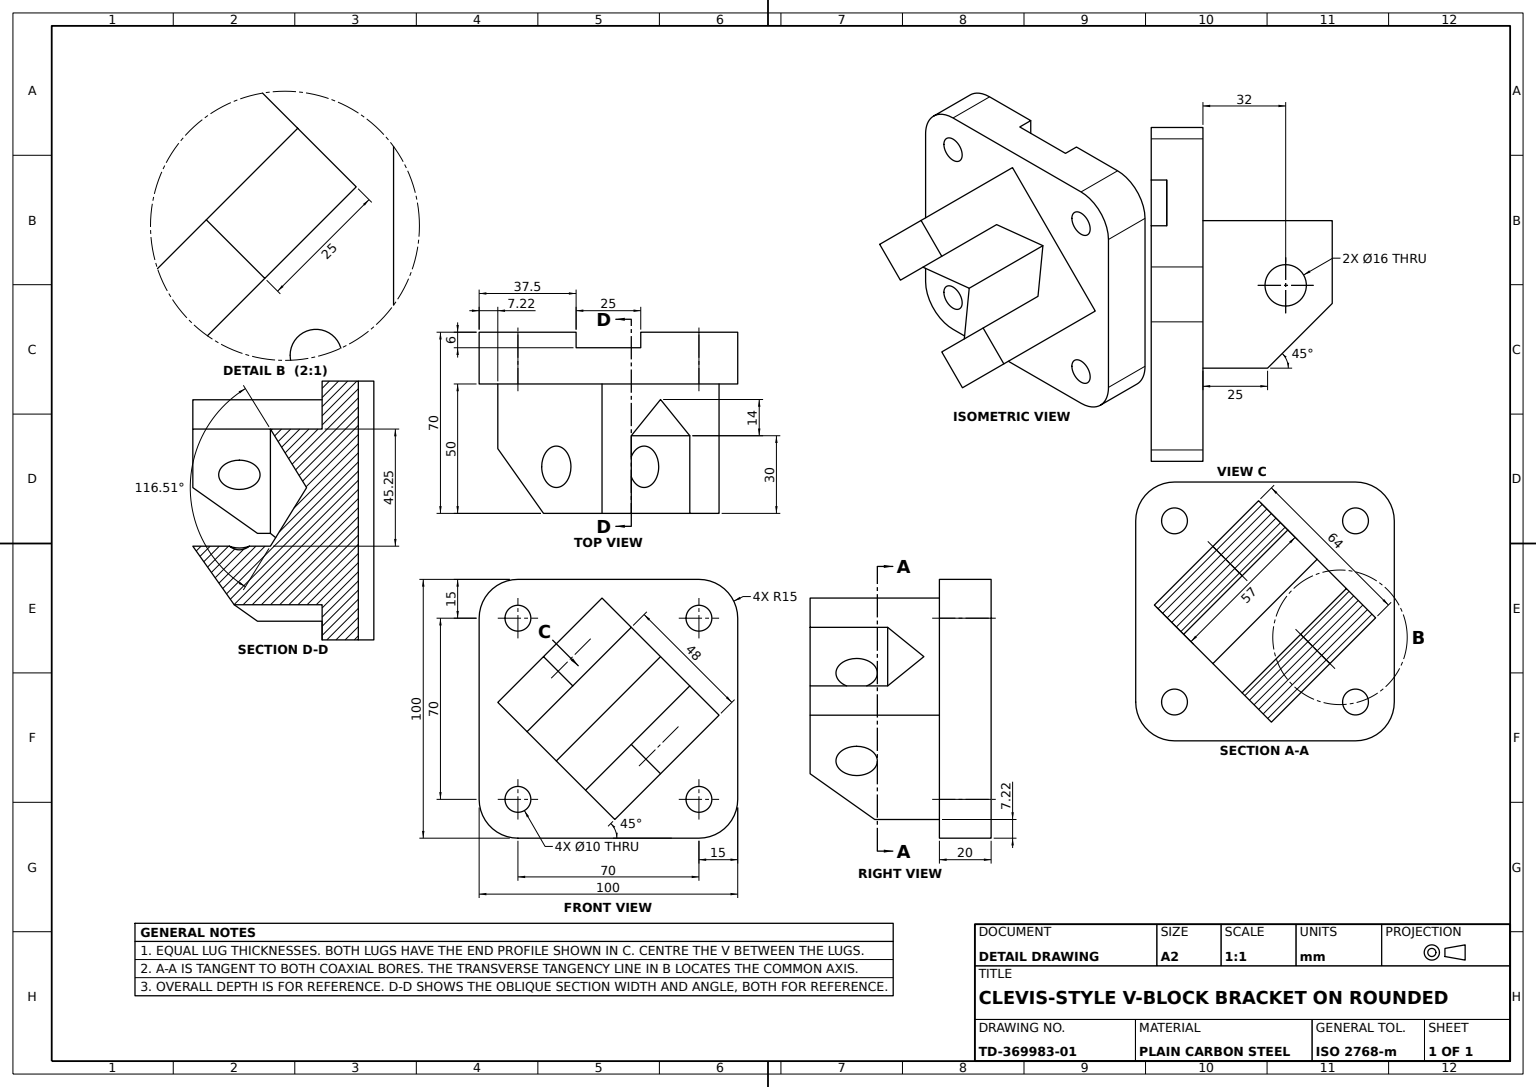
from build123d import *

# Parameters (mm, degrees)
BASE_PLATE_SKETCH_R       = 5
BASE_PLATE_DEPTH          = 20
PLATE_HOLES_12_DEPTH      = 114.578166916
PLATE_HOLES_12_DEPTH_BACK = 114.578166916
PLATE_HOLES_SKETCH_W      = 25
PLATE_HOLES_SKETCH_H      = 12
SQUARE_BOSS_DEPTH         = 50
BOSS_HOLE_16_DEPTH        = 125.295950858
BOSS_HOLE_16_DEPTH_BACK   = 125.295950858
BOSS_HOLE_SKETCH_R        = 8
BOSS_CHAMFER_25X45_SIZE   = 25
SLOT_CUT_DEPTH            = 122.4197622
SLOT_CUT_DEPTH_BACK       = 122.4197622


with BuildPart() as part:
    # Base Plate Sketch → Base Plate (new body)
    with BuildSketch(Plane.XY):
        with BuildLine():
            Line((-35, 50), (35, 50))
            ThreePointArc((35, 50), (45.606601718, 45.606601718), (50, 35))
            Line((50, 35), (50, -35))
            ThreePointArc((50, -35), (45.606601718, -45.606601718), (35, -50))
            Line((35, -50), (-35, -50))
            ThreePointArc((-35, -50), (-45.606601718, -45.606601718), (-50, -35))
            Line((-50, -35), (-50, 35))
            ThreePointArc((-50, 35), (-45.606601718, 45.606601718), (-35, 50))
        make_face()
        with Locations((-35, 35)):
            Circle(BASE_PLATE_SKETCH_R, mode=Mode.SUBTRACT)
        with Locations((35, 35)):
            Circle(BASE_PLATE_SKETCH_R, mode=Mode.SUBTRACT)
        with Locations((35, -35)):
            Circle(BASE_PLATE_SKETCH_R, mode=Mode.SUBTRACT)
        with Locations((-35, -35)):
            Circle(BASE_PLATE_SKETCH_R, mode=Mode.SUBTRACT)
    extrude(amount=BASE_PLATE_DEPTH)

    # Plate Holes Sketch → Plate Holes Ø12 (cut, two sides: drawn at the far end of the back side and taken through both)
    with BuildSketch(Plane.XZ.offset(50).offset(-PLATE_HOLES_12_DEPTH_BACK)):
        Rectangle(PLATE_HOLES_SKETCH_W, PLATE_HOLES_SKETCH_H)
    extrude(amount=PLATE_HOLES_12_DEPTH + PLATE_HOLES_12_DEPTH_BACK, mode=Mode.SUBTRACT)

    # Square Boss Sketch → Square Boss (add)
    with BuildSketch(Plane.XY.offset(20)):
        Polygon((-42.779960262, 2.474873734), (-2.474873734, 42.779960262), (42.779960262, -2.474873734), (2.474873734, -42.779960262), align=None)
    extrude(amount=SQUARE_BOSS_DEPTH)

    # Boss Hole Sketch → Boss Hole Ø16 (cut, two sides: drawn at the far end of the back side and taken through both)
    with BuildSketch(Plane(origin=(22.627416998, -22.627416998, 0), x_dir=(0, 0, -1), z_dir=(0.7071067811865462, -0.7071067811865488, 0)).offset(-BOSS_HOLE_16_DEPTH_BACK)):
        with Locations(Location((-52, 3.5, 0), (0, 0, 90))):
            Circle(BOSS_HOLE_SKETCH_R)
    extrude(amount=BOSS_HOLE_16_DEPTH + BOSS_HOLE_16_DEPTH_BACK, mode=Mode.SUBTRACT)

    # Boss Chamfer 25x45°
    boss_chamfer_25x45_edges = [part.edges().sort_by_distance(p)[0] for p in [
        (-20.152543264, -20.152543264, 70),
    ]]
    chamfer(boss_chamfer_25x45_edges, length=BOSS_CHAMFER_25X45_SIZE)

    # Slot Sketch → Slot Cut (cut, two sides: drawn at the far end of the back side and taken through both)
    with BuildSketch(Plane(origin=(20.152543264, 20.152543264, 0), x_dir=(0, 0, -1), z_dir=(0.7071067811865486, 0.7071067811865465, 0)).offset(-SLOT_CUT_DEPTH_BACK)):
        Polygon((-70, 16), (-40, 16), (-26, 0), (-40, -16), (-70, -16), align=None)
    extrude(amount=SLOT_CUT_DEPTH + SLOT_CUT_DEPTH_BACK, mode=Mode.SUBTRACT)


solid = part.part
